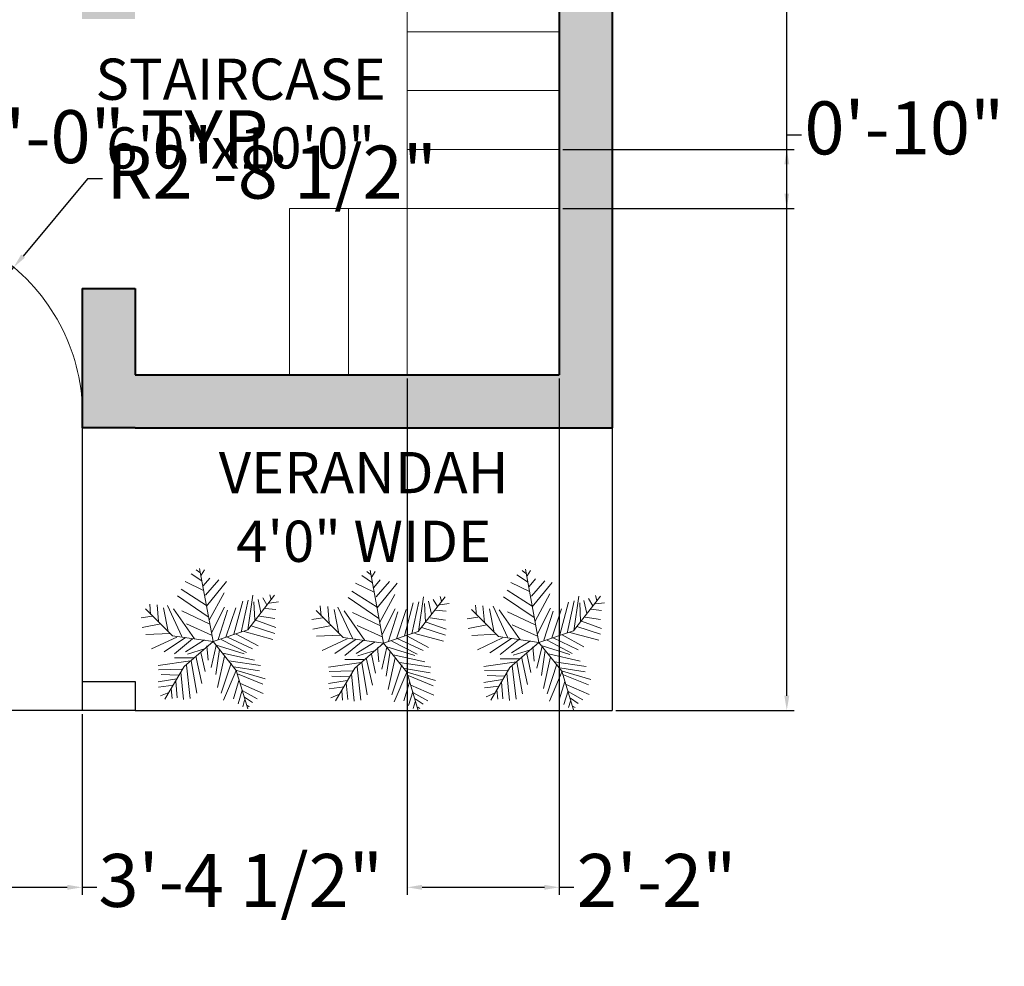
# Model space of a CAD drawing. Units: inches. Extents: x 1883 to 2353, y 1976 to 2541.
# Tile 3 of 5: x 2170 to 2337, y 1976 to 2136. Entities that reach past the tile are written whole.
import ezdxf

# ---------------------------------------------------------------- set-up
doc = ezdxf.new("R2010")
doc.units = ezdxf.units.IN
for name, color, linetype, lineweight in [('A-ANNO-DIMS', 2, 'Continuous', 18), ('A-AREA-IDEN', 7, 'Continuous', 18), ('A-DOOR', 3, 'Continuous', 18), ('A-FLOR-OTLN', 7, 'Continuous', 25), ('A-FLOR-STRS', 7, 'Continuous', 18), ('A-WALL', 7, 'Continuous', 40), ('C-SITE', 7, 'Continuous', 25), ('L-PLNT', 94, 'Continuous', 13)]:
    doc.layers.add(name, color=color, linetype=linetype, lineweight=lineweight)
doc.layers.add('A-WALL-PATT', color=67, linetype='Continuous', lineweight=13, true_color=0x727430)
doc.styles.get("Standard").update_dxf_attribs({"font": 'arial.ttf'})
doc.dimstyles.new('ISO-25', dxfattribs={"dimtxt": 9, "dimasz": 2.5, "dimexe": 1.25, "dimexo": 0.625, "dimgap": 2, "dimtad": 0, "dimtih": 1, "dimtoh": 1, "dimdec": 1, "dimlunit": 4, "dimtxsty": 'Standard', "dimcen": 2.5, "dimadec": 0, "dimazin": 0, "dimtfac": 1, "dimtdec": 1, "dimtmove": 0, "dimatfit": 3, "dimfxl": 1, "dimarcsym": 0})

# ---------------------------------------------------------------- blocks, each defined once
blk = doc.blocks.new('*U12')
for p, q in [((-10.186, 53.64), (-13.084, 55.962)), ((0, 0), (-10.5, 57)), ((-9.099, 51.782), (-6.563, 55.962)), ((-7.288, 39.707), (-21.778, 46.673)), ((-8.737, 47.138), (-17.069, 52.711)), ((-7.65, 43.423), (-2.578, 49.46)), ((-5.839, 35.992), (4.667, 48.067)), ((-5.114, 27.632), (10.463, 46.673)), ((-5.114, 28.097), (-24.676, 40.636)), ((-3.665, 19.273), (-27.574, 35.527)), ((-2.941, 16.486), (8.652, 37.85)), ((16.259, 5.805), (23.142, 31.348)), ((22.055, 7.198), (27.489, 32.277)), ((27, 9), (48, 36)), ((27.127, 9.056), (31.112, 35.992)), ((31.836, 30.883), (32.561, 16.486)), ((35.096, 32.741), (37.27, 22.524)), ((38.719, 34.134), (41.979, 28.561)), ((43.791, 29.954), (51.036, 30.883)), ((44.153, 36.456), (45.239, 32.741)), ((-31.5, 4.5), (-52.5, 25.5)), ((-48.585, 21.131), (-49.309, 29.026)), ((-43.513, 28.561), (-42.427, 15.558)), ((-38.442, 26.239), (-34.819, 7.663)), ((-35.544, 28.097), (-24.314, 3.947)), ((-14.533, 2.09), (-30.834, 25.31)), ((-24.314, 23.917), (-2.941, 13.7)), ((-1.129, 6.734), (9.014, 26.704)), ((3.942, 1.625), (11.187, 24.381)), ((10.101, 3.483), (17.708, 26.239)), ((40.53, 25.775), (48.862, 24.846)), ((-47.498, 19.737), (-55.83, 18.344)), ((33.285, 16.486), (48.862, 10.913)), ((36.183, 19.737), (48.137, 17.88)), ((-40.615, 13.7), (-55.105, 10.913)), ((-20.691, 13.7), (-1.129, 4.876)), ((0, 0), (27, 9)), ((29.662, 12.307), (48.137, 6.269)), ((-33.37, 6.269), (-52.207, 5.34)), ((-28.299, 3.483), (-47.86, -5.805)), ((-21.416, 3.018), (-38.079, -8.128)), ((0, 0), (-31.5, 4.5)), ((-15.982, 2.09), (-30.11, -9.521)), ((0, 0), (-22.5, -19.5)), ((-6.563, 1.161), (-21.416, -8.128)), ((0, 0), (18, -22.5)), ((6.478, 1.625), (26.04, -8.592)), ((11.187, 3.483), (30.749, -5.805)), ((18.07, 5.805), (35.096, -3.483)), ((24.229, 7.663), (46.688, 1.625)), ((-6.563, -5.805), (-19.967, -9.985)), ((-4.752, -3.483), (-3.665, -14.629)), ((2.493, -3.019), (-1.491, -20.202)), ((1.769, -2.555), (24.229, -9.521)), ((5.029, -6.27), (2.131, -25.775)), ((-17.431, -15.094), (-42.789, -18.809)), ((-15.257, -12.772), (-30.11, -12.772)), ((-17.069, -15.094), (-12.721, -40.172)), ((-13.446, -11.378), (-8.737, -32.741)), ((-9.461, -8.592), (-6.201, -23.453)), ((9.014, -11.378), (3.58, -35.992)), ((7.565, -9.056), (32.198, -14.629)), ((12.274, -15.094), (36.907, -18.809)), ((-24.314, -21.596), (-42.427, -22.06)), ((-22.5, -19.5), (-37.5, -45)), ((-20.691, -18.345), (-17.793, -44.352)), ((14.085, -16.951), (6.478, -40.172)), ((18.07, -22.524), (8.289, -45.745)), ((16.259, -19.738), (36.183, -22.989)), ((18, -22.5), (27, -52.5)), ((18.433, -22.524), (40.53, -29.026)), ((-28.299, -29.026), (-42.789, -31.348)), ((-26.849, -26.24), (-40.253, -25.775)), ((-25.038, -23.918), (-22.865, -45.281)), ((20.244, -30.419), (15.897, -44.816)), ((19.157, -25.311), (38.719, -33.206)), ((-30.834, -34.135), (-42.427, -35.528)), ((-32.646, -36.921), (-31.921, -44.352)), ((-29.023, -30.884), (-27.936, -43.887)), ((22.78, -37.85), (19.519, -48.532)), ((21.331, -32.741), (39.081, -40.636)), ((22.78, -38.314), (34.372, -44.816)), ((-34.457, -39.708), (-40.978, -42.494)), ((24.591, -45.745), (23.142, -50.854)), ((24.591, -43.423), (30.749, -47.603)), ((26.764, -49.925), (28.213, -50.854))]:
    blk.add_line(p, q)
blk = doc.blocks.new('*D21')
at = {"layer": 'A-ANNO-DIMS', "color": 0, "lineweight": -2, "transparency": 16777216}
for p, q in [((2051.49, 2121.95), (2051.49, 2114.12)), ((2099.49, 2121.95), (2099.49, 2114.12)), ((2053.99, 2115.37), (2096.99, 2115.37)), ((2099.49, 2115.37), (2101.99, 2115.37))]:
    blk.add_line(p, q, dxfattribs=at)
at = {"layer": 'A-ANNO-DIMS', "color": 0, "transparency": 16777216}
for points in [[(2053.99, 2115.79), (2053.99, 2114.96), (2051.49, 2115.37)], [(2096.99, 2115.79), (2096.99, 2114.96), (2099.49, 2115.37)]]:
    blk.add_solid(points, dxfattribs=at)
at = {"layer": 'Defpoints', "color": 0, "transparency": 16777216}
for p in [(2051.49, 2122.57), (2099.49, 2122.57), (2099.49, 2115.37)]:
    blk.add_point(p, dxfattribs=at)
at = {"layer": 'A-ANNO-DIMS', "color": 0, "transparency": 16777216, "insert": (2160.94, 2115.37), "char_height": 9, "attachment_point": 5}
blk.add_mtext('WINDOW 4\'-0" TYP.', dxfattribs=at)
blk = doc.blocks.new('*D43')
at = {"layer": 'A-ANNO-DIMS', "color": 0, "lineweight": -2, "transparency": 16777216}
for p, q in [((2271.12, 2502.07), (2301.39, 2502.07)), ((2300.14, 2499.57), (2300.14, 2267.17)), ((2300.14, 2021.57), (2300.14, 2253.97)), ((2271.12, 2019.07), (2301.39, 2019.07))]:
    blk.add_line(p, q, dxfattribs=at)
at = {"layer": 'A-ANNO-DIMS', "color": 0, "transparency": 16777216}
for points in [[(2299.73, 2499.57), (2300.56, 2499.57), (2300.14, 2502.07)], [(2299.73, 2021.57), (2300.56, 2021.57), (2300.14, 2019.07)]]:
    blk.add_solid(points, dxfattribs=at)
at = {"layer": 'Defpoints', "color": 0, "transparency": 16777216}
for p in [(2270.49, 2502.07), (2300.14, 2502.07), (2270.49, 2019.07)]:
    blk.add_point(p, dxfattribs=at)
at = {"layer": 'A-ANNO-DIMS', "color": 0, "transparency": 16777216, "insert": (2300.14, 2260.57), "char_height": 9, "attachment_point": 5}
blk.add_mtext('40\'-3"', dxfattribs=at)
blk = doc.blocks.new('*D45')
at = {"layer": 'A-ANNO-DIMS', "color": 0, "lineweight": -2, "transparency": 16777216}
for p, q in [((2139.99, 2018.45), (2139.99, 1987.78)), ((2180.49, 2018.45), (2180.49, 1987.78)), ((2142.49, 1989.03), (2177.99, 1989.03)), ((2180.49, 1989.03), (2182.99, 1989.03))]:
    blk.add_line(p, q, dxfattribs=at)
at = {"layer": 'A-ANNO-DIMS', "color": 0, "transparency": 16777216}
for points in [[(2142.49, 1989.45), (2142.49, 1988.61), (2139.99, 1989.03)], [(2177.99, 1989.45), (2177.99, 1988.61), (2180.49, 1989.03)]]:
    blk.add_solid(points, dxfattribs=at)
at = {"layer": 'Defpoints', "color": 0, "transparency": 16777216}
for p in [(2139.99, 2019.07), (2180.49, 2019.07), (2180.49, 1989.03)]:
    blk.add_point(p, dxfattribs=at)
at = {"layer": 'A-ANNO-DIMS', "color": 0, "transparency": 16777216, "insert": (2207.44, 1989.03), "char_height": 9, "attachment_point": 5}
blk.add_mtext('3\'-4 1/2"', dxfattribs=at)
blk = doc.blocks.new('*D52')
at = {"layer": 'A-ANNO-DIMS', "color": 0, "lineweight": -2, "transparency": 16777216}
for p, q in [((2300.14, 2114.36), (2300.14, 2116.86)), ((2300.14, 2116.86), (2302.64, 2116.86)), ((2262.12, 2114.36), (2301.39, 2114.36)), ((2300.14, 2106.86), (2300.14, 2111.86)), ((2262.12, 2104.36), (2301.39, 2104.36))]:
    blk.add_line(p, q, dxfattribs=at)
at = {"layer": 'A-ANNO-DIMS', "color": 0, "transparency": 16777216}
for points in [[(2299.73, 2111.86), (2300.56, 2111.86), (2300.14, 2114.36)], [(2299.73, 2106.86), (2300.56, 2106.86), (2300.14, 2104.36)]]:
    blk.add_solid(points, dxfattribs=at)
at = {"layer": 'Defpoints', "color": 0, "transparency": 16777216}
for p in [(2261.49, 2114.36), (2300.14, 2114.36), (2261.49, 2104.36)]:
    blk.add_point(p, dxfattribs=at)
at = {"layer": 'A-ANNO-DIMS', "color": 0, "transparency": 16777216, "insert": (2320.1, 2116.86), "char_height": 9, "attachment_point": 5}
blk.add_mtext('0\'-10"', dxfattribs=at)
blk = doc.blocks.new('*D53')
at = {"layer": 'A-ANNO-DIMS', "color": 0, "lineweight": -2, "transparency": 16777216}
for p, q in [((2235.72, 2075.45), (2235.72, 1987.78)), ((2261.49, 2075.45), (2261.49, 1987.78)), ((2238.22, 1989.03), (2258.99, 1989.03)), ((2261.49, 1989.03), (2263.99, 1989.03))]:
    blk.add_line(p, q, dxfattribs=at)
at = {"layer": 'A-ANNO-DIMS', "color": 0, "transparency": 16777216}
for points in [[(2238.22, 1989.45), (2238.22, 1988.61), (2235.72, 1989.03)], [(2258.99, 1989.45), (2258.99, 1988.61), (2261.49, 1989.03)]]:
    blk.add_solid(points, dxfattribs=at)
at = {"layer": 'Defpoints', "color": 0, "transparency": 16777216}
for p in [(2235.72, 2076.07), (2261.49, 2076.07), (2261.49, 1989.03)]:
    blk.add_point(p, dxfattribs=at)
at = {"layer": 'A-ANNO-DIMS', "color": 0, "transparency": 16777216, "insert": (2278.03, 1989.03), "char_height": 9, "attachment_point": 5}
blk.add_mtext('2\'-2"', dxfattribs=at)
blk = doc.blocks.new('*D61')
at = {"layer": 'A-ANNO-DIMS', "color": 0, "lineweight": -2, "transparency": 16777216}
for p, q in [((2181.45, 2109.35), (2170.49, 2096.26)), ((2183.95, 2109.35), (2181.45, 2109.35)), ((2147.95, 2069.32), (2168.88, 2094.34))]:
    blk.add_line(p, q, dxfattribs=at)
at = {"layer": 'A-ANNO-DIMS', "color": 0, "transparency": 16777216}
blk.add_solid([(2170.17, 2096.53), (2170.81, 2095.99), (2168.88, 2094.34)], dxfattribs=at)
at = {"layer": 'Defpoints', "color": 0, "transparency": 16777216}
for p in [(2168.88, 2094.34), (2147.95, 2069.32)]:
    blk.add_point(p, dxfattribs=at)
at = {"layer": 'A-ANNO-DIMS', "color": 0, "transparency": 16777216, "insert": (2212.7, 2109.35), "char_height": 9, "attachment_point": 5}
blk.add_mtext('R2\'-8 1/2"', dxfattribs=at)

msp = doc.modelspace()

# ---------------------------------------------------------------- hatches: boundary and pattern name
at = {"layer": 'A-WALL-PATT'}
h = msp.add_hatch(color=256, dxfattribs=at)
h.dxf.hatch_style = 1
h.paths.add_polyline_path([(2189.49, 2090.74), (2180.49, 2090.74), (2180.49, 2071.57, -0.034524), (2180.49, 2067.07), (2189.49, 2067.07), (2261.49, 2067.07), (2270.49, 2067.07), (2270.49, 2094.07), (2270.49, 2255.69), (2261.49, 2255.69), (2261.49, 2200.57), (2261.49, 2196.07), (2261.49, 2094.07), (2261.49, 2076.07), (2189.49, 2076.07)])
h.paths.add_polyline_path([(2189.49, 2196.07), (2208.94, 2196.07), (2208.94, 2200.57), (2151.99, 2200.57), (2139.99, 2200.57), (2139.99, 2251.57), (2139.99, 2256.07), (2135.49, 2256.07), (2134.13, 2256.07), (2134.13, 2251.57), (2135.49, 2251.57), (2135.49, 2131.57), (2099.49, 2131.57), (2099.49, 2122.57), (2103.99, 2122.57), (2135.49, 2122.57), (2139.99, 2122.57), (2139.99, 2196.07), (2151.99, 2196.07), (2180.49, 2196.07), (2180.49, 2136.51), (2189.49, 2136.51)])

# ---------------------------------------------------------------- linework, layer by layer
at = {"layer": 'A-DOOR'}
msp.add_arc((2147.95, 2069.32), 32.63, 356.0455, 104.1079, dxfattribs=at)
at = {"layer": 'A-FLOR-OTLN'}
for p, q in [((2180.49, 2067.07), (2180.49, 2023.99)), ((2270.49, 2067.07), (2270.49, 2019.07)), ((2180.49, 2023.99), (2189.49, 2023.99)), ((2180.49, 2023.99), (2180.49, 2019.07)), ((2189.49, 2023.99), (2189.49, 2019.07)), ((2189.49, 2019.07), (2180.49, 2019.07)), ((2189.49, 2019.07), (2261.49, 2019.07)), ((2261.49, 2019.07), (2270.49, 2019.07))]:
    msp.add_line(p, q, dxfattribs=at)
at = {"layer": 'A-FLOR-STRS'}
for p, q in [((2235.72, 2221.83), (2235.72, 2104.36)), ((2235.72, 2134.36), (2261.49, 2134.36)), ((2235.72, 2124.36), (2261.49, 2124.36)), ((2235.72, 2114.36), (2261.49, 2114.36)), ((2215.72, 2104.36), (2215.72, 2076.07)), ((2235.72, 2104.36), (2215.72, 2104.36)), ((2225.72, 2104.36), (2225.72, 2076.07)), ((2235.72, 2104.36), (2261.49, 2104.36)), ((2235.72, 2104.36), (2235.72, 2076.07))]:
    msp.add_line(p, q, dxfattribs=at)
at = {"layer": 'A-WALL'}
for p, q in [((2270.49, 2502.07), (2270.49, 2094.07)), ((2261.49, 2196.07), (2261.49, 2094.07)), ((2261.49, 2094.07), (2261.49, 2076.07)), ((2270.49, 2094.07), (2270.49, 2067.07)), ((2180.49, 2090.74), (2180.49, 2071.57)), ((2180.49, 2090.74), (2189.49, 2090.74)), ((2189.49, 2090.74), (2189.49, 2076.07)), ((2189.49, 2076.07), (2261.49, 2076.07)), ((2180.49, 2071.57), (2180.49, 2067.07)), ((2189.49, 2067.07), (2180.49, 2067.07)), ((2189.49, 2067.07), (2261.49, 2067.07)), ((2261.49, 2067.07), (2270.49, 2067.07))]:
    msp.add_line(p, q, dxfattribs=at)
at = {"layer": 'C-SITE'}
msp.add_line((2180.49, 2019.07), (2006.49, 2019.07), dxfattribs=at)

# ---------------------------------------------------------------- block references
at = {"layer": 'L-PLNT', "xscale": 0.2179590827651691, "yscale": 0.2179590827651691, "zscale": 0.2179590827651691}
for p in [(2202.73, 2030.79), (2231.69, 2030.5), (2258.05, 2030.64)]:
    msp.add_blockref('*U12', p, dxfattribs=at)

# ---------------------------------------------------------------- texts
at = {"layer": 'A-AREA-IDEN', "char_height": 7, "attachment_point": 1}
for s, width, insert in [('\\pxqc;{\\fArial|b1|i0|c0|p34;STAIRCASE\\P6\'0"x10\'0"}', 46.7836, (2184.03, 2129.8)), ('\\pxqc;{\\fArial|b1|i0|c0|p34;VERANDAH\\P4\'0" WIDE}', 64.9328, (2195.85, 2062.98))]:
    msp.add_mtext_dynamic_manual_height_columns(s, width=width, gutter_width=12.5, heights=[0], dxfattribs=dict(at, insert=insert))

# ---------------------------------------------------------------- dimensions: what is measured, and where the dimension line sits
at = {"layer": 'A-ANNO-DIMS'}
for base, p1, p2, picture, middle in [((2300.14, 2502.07), (2270.49, 2019.07), (2270.49, 2502.07), '*D43', (2300.14, 2260.57)), ((2300.14, 2114.36), (2261.49, 2104.36), (2261.49, 2114.36), '*D52', (2320.1, 2116.86))]:
    dim = msp.add_linear_dim(base=base, p1=p1, p2=p2, angle=90, dimstyle='ISO-25', override={"dimdec": 1, "dimlfac": 1, "dimrnd": 0, "dimzin": 1, "dimdsep": 46, "dimlunit": 4, "dimfrac": 2}, dxfattribs=at)
    dim.commit()
    dim.dimension.update_dxf_attribs({"geometry": picture, "text_midpoint": middle})
dim = msp.add_linear_dim(base=(2099.49, 2115.37), p1=(2051.49, 2122.57), p2=(2099.49, 2122.57), text='WINDOW <> TYP.', dimstyle='ISO-25', override={"dimdec": 1, "dimlfac": 1, "dimrnd": 0, "dimzin": 1, "dimdsep": 46, "dimlunit": 4, "dimfrac": 2}, dxfattribs=at)
dim.commit()
dim.dimension.update_dxf_attribs({"geometry": '*D21', "text_midpoint": (2160.94, 2115.37)})
dim = msp.add_radius_dim(center=(2147.95, 2069.32), mpoint=(2168.88, 2094.34), dimstyle='ISO-25', override={"dimdec": 1, "dimlfac": 1, "dimrnd": 0, "dimzin": 1, "dimdsep": 46, "dimlunit": 4, "dimfrac": 2}, dxfattribs=at)
dim.commit()
dim.dimension.update_dxf_attribs({"geometry": '*D61', "text_midpoint": (2212.7, 2109.35), "dimtype": 164})
for base, p1, p2, picture, middle in [((2261.49, 1989.03), (2235.72, 2076.07), (2261.49, 2076.07), '*D53', (2278.03, 1989.03)), ((2180.49, 1989.03), (2139.99, 2019.07), (2180.49, 2019.07), '*D45', (2207.44, 1989.03))]:
    dim = msp.add_linear_dim(base=base, p1=p1, p2=p2, dimstyle='ISO-25', override={"dimdec": 1, "dimlfac": 1, "dimrnd": 0, "dimzin": 1, "dimdsep": 46, "dimlunit": 4, "dimfrac": 2}, dxfattribs=at)
    dim.commit()
    dim.dimension.update_dxf_attribs({"geometry": picture, "text_midpoint": middle})

doc.saveas('drawing.dxf')
